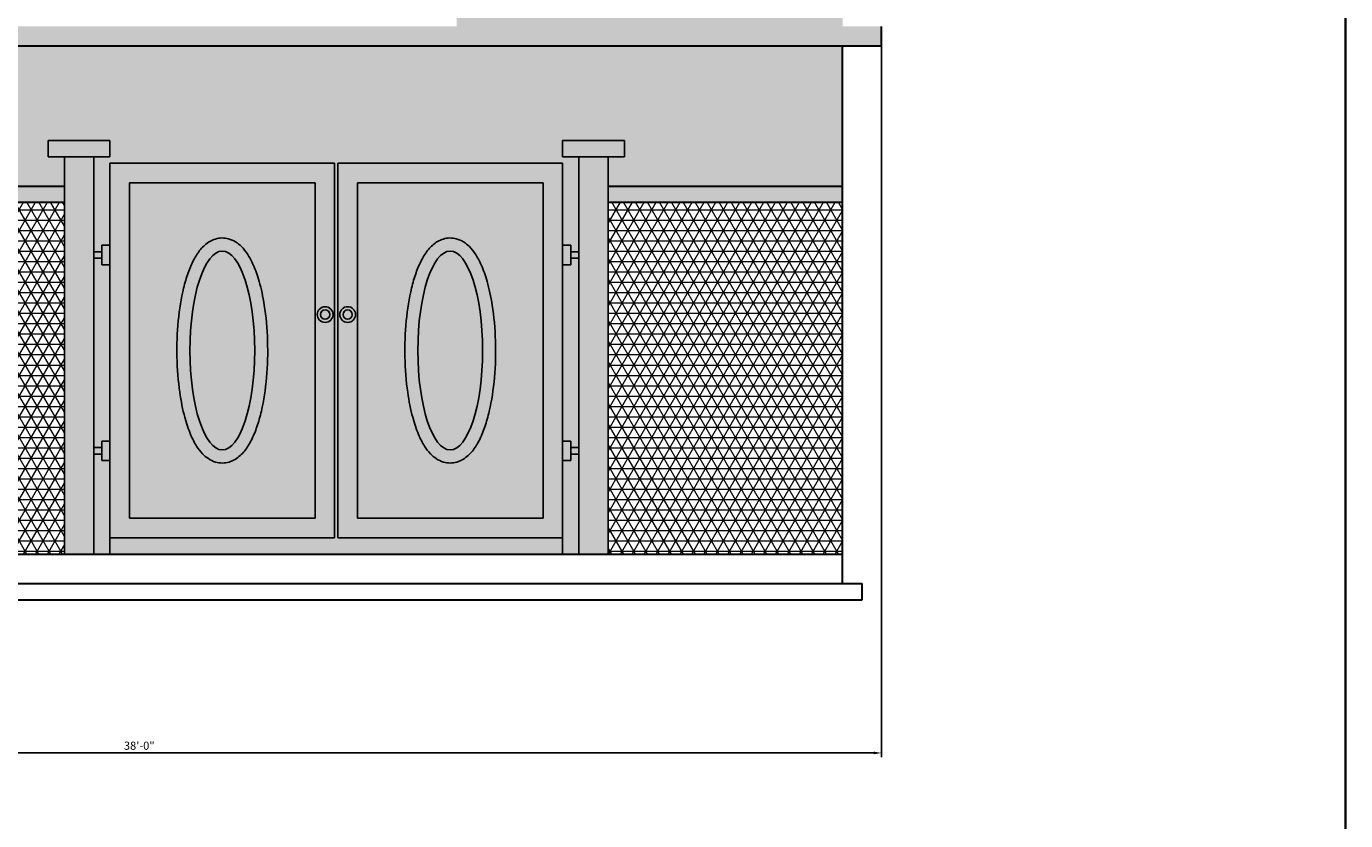
# Model space of a CAD drawing. Units: inches. Extents: x 2391 to 16591, y 7259 to 10239.
# Tile 12 of 27: x 3749 to 4154, y 7502 to 7746. Entities that reach past the tile are written whole.
import ezdxf

# ---------------------------------------------------------------- set-up
doc = ezdxf.new("R2010")
doc.units = ezdxf.units.IN
for name, color, linetype, lineweight in [('A-ANNO-DIMS', 4, 'Continuous', 18), ('A-ANNO-TTLB', 7, 'Continuous', 35), ('A-ELEV', 7, 'Continuous', 30), ('A-ELEV-GATE', 7, 'Continuous', 25), ('A-ELEV-GATE-PATT', 252, 'Continuous', 13), ('A-ELEV-PATT', 8, 'Continuous', 13), ('A-ELEV-SURF-PATT', 253, 'Continuous', 13)]:
    doc.layers.add(name, color=color, linetype=linetype, lineweight=lineweight)
doc.styles.get("Standard").update_dxf_attribs({"font": 'arial.ttf'})
doc.dimstyles.new('ISO-25', dxfattribs={"dimtxt": 2.5, "dimasz": 2.5, "dimexe": 1.25, "dimexo": 0.625, "dimtad": 1, "dimdec": 0, "dimlunit": 3, "dimtxsty": 'Standard', "dimcen": 2.5, "dimadec": 0, "dimazin": 0, "dimtfac": 1, "dimtdec": 0, "dimtmove": 0, "dimatfit": 3, "dimfxl": 1, "dimarcsym": 0})

# ---------------------------------------------------------------- blocks, each defined once
blk = doc.blocks.new('*D91')
at = {"layer": 'A-ANNO-DIMS', "color": 0, "lineweight": -2, "transparency": 16777216}
for p, q in [((3555.71, 7745.56), (3555.71, 7521.88)), ((4011.71, 7745.56), (4011.71, 7521.88)), ((3558.21, 7523.13), (4009.21, 7523.13))]:
    blk.add_line(p, q, dxfattribs=at)
at = {"layer": 'A-ANNO-DIMS', "color": 0, "transparency": 16777216}
for points in [[(3558.21, 7523.55), (3558.21, 7522.71), (3555.71, 7523.13)], [(4009.21, 7523.55), (4009.21, 7522.71), (4011.71, 7523.13)]]:
    blk.add_solid(points, dxfattribs=at)
at = {"layer": 'Defpoints', "color": 0, "transparency": 16777216}
for p in [(3555.71, 7746.18), (4011.71, 7746.18), (4011.71, 7523.13)]:
    blk.add_point(p, dxfattribs=at)
at = {"layer": 'A-ANNO-DIMS', "color": 0, "transparency": 16777216, "insert": (3783.71, 7525.03), "char_height": 2.5, "attachment_point": 5}
blk.add_mtext('38\'-0"', dxfattribs=at)
blk = doc.blocks.new('*D92')
at = {"layer": 'A-ANNO-DIMS', "color": 0, "lineweight": -2, "transparency": 16777216}
for p, q in [((3777.58, 8333.18), (3507.41, 8333.18)), ((3508.66, 7572.68), (3508.66, 8330.68)), ((3561.08, 7570.18), (3507.41, 7570.18))]:
    blk.add_line(p, q, dxfattribs=at)
at = {"layer": 'A-ANNO-DIMS', "color": 0, "transparency": 16777216}
for points in [[(3508.24, 8330.68), (3509.08, 8330.68), (3508.66, 8333.18)], [(3508.24, 7572.68), (3509.08, 7572.68), (3508.66, 7570.18)]]:
    blk.add_solid(points, dxfattribs=at)
at = {"layer": 'Defpoints', "color": 0, "transparency": 16777216}
for p in [(3508.66, 8333.18), (3778.21, 8333.18), (3561.71, 7570.18)]:
    blk.add_point(p, dxfattribs=at)
at = {"layer": 'A-ANNO-DIMS', "color": 0, "transparency": 16777216, "insert": (3506.76, 7951.68), "char_height": 2.5, "attachment_point": 5, "rotation": 90}
blk.add_mtext('63\'-7"', dxfattribs=at)

msp = doc.modelspace()

# ---------------------------------------------------------------- hatches: boundary and pattern name
at = {"layer": 'A-ELEV-GATE-PATT'}
h = msp.add_hatch(color=256, dxfattribs=at)
h.dxf.hatch_style = 1
h.paths.add_polyline_path([(3760.71, 7584.18), (3769.71, 7584.18), (3769.71, 7706.18), (3760.71, 7706.18)])
h.paths.add_polyline_path([(3927.71, 7706.18), (3918.71, 7706.18), (3918.71, 7584.18), (3927.71, 7584.18)])
h = msp.add_hatch(color=256, dxfattribs=at)
h.dxf.hatch_style = 1
h.paths.add_polyline_path([(3774.71, 7589.18), (3843.71, 7589.18), (3843.71, 7704.18), (3774.71, 7704.18)])
h.paths.add_polyline_path([(3780.71, 7698.18), (3837.71, 7698.18), (3837.71, 7595.18), (3780.71, 7595.18)], flags=16)
edge = h.paths.add_edge_path(flags=0)
edge.add_spline(control_points=[(3809.21, 7612.14), (3809.91, 7612.14), (3810.62, 7612.25), (3811.94, 7612.64), (3812.56, 7612.92), (3813.7, 7613.59), (3814.21, 7613.98), (3815.17, 7614.84), (3815.6, 7615.31), (3816.82, 7616.8), (3817.52, 7617.93), (3818.78, 7620.42), (3819.34, 7621.79), (3820.36, 7624.75), (3820.81, 7626.35), (3821.94, 7631.21), (3822.47, 7634.72), (3823.12, 7642.05), (3823.22, 7645.88), (3822.99, 7653.42), (3822.66, 7657.13), (3821.7, 7663.19), (3821.18, 7665.65), (3820.01, 7669.74), (3819.41, 7671.44), (3818.18, 7674.2), (3817.58, 7675.32), (3816.36, 7677.16), (3815.76, 7677.91), (3814.54, 7679.12), (3813.94, 7679.61), (3812.61, 7680.43), (3811.87, 7680.77), (3810.43, 7681.15), (3809.76, 7681.23), (3808.41, 7681.21), (3807.74, 7681.1), (3806.48, 7680.72), (3805.88, 7680.46), (3804.79, 7679.82), (3804.29, 7679.45), (3803.37, 7678.64), (3802.95, 7678.2), (3801.74, 7676.76), (3801.04, 7675.67), (3799.78, 7673.25), (3799.21, 7671.92), (3798.19, 7669.04), (3797.74, 7667.49), (3796.6, 7662.76), (3796.04, 7659.34), (3795.35, 7652.17), (3795.21, 7648.41), (3795.36, 7640.98), (3795.65, 7637.3), (3796.53, 7631.12), (3797.05, 7628.54), (3798.2, 7624.26), (3798.8, 7622.48), (3800.03, 7619.59), (3800.63, 7618.41), (3801.85, 7616.48), (3802.45, 7615.7), (3803.67, 7614.43), (3804.26, 7613.91), (3805.6, 7613.04), (3806.34, 7612.67), (3807.81, 7612.25), (3808.51, 7612.14), (3809.21, 7612.14)], knot_values=[0, 0, 0, 0, 0.095196, 0.095196, 0.190392, 0.190392, 0.285588, 0.285588, 0.380784, 0.380784, 0.570897, 0.570897, 0.76101, 0.76101, 0.951123, 0.951123, 1.307609, 1.307609, 1.664096, 1.664096, 2.020583, 2.020583, 2.290036, 2.290036, 2.5108, 2.5108, 2.687191, 2.687191, 2.829292, 2.829292, 2.942747, 2.942747, 3.056202, 3.056202, 3.147245, 3.147245, 3.238288, 3.238288, 3.329331, 3.329331, 3.420374, 3.420374, 3.511418, 3.511418, 3.698581, 3.698581, 3.885745, 3.885745, 4.072908, 4.072908, 4.42383, 4.42383, 4.774752, 4.774752, 5.125674, 5.125674, 5.403289, 5.403289, 5.629501, 5.629501, 5.810378, 5.810378, 5.956164, 5.956164, 6.072402, 6.072402, 6.18864, 6.18864, 6.283185, 6.283185, 6.283185, 6.283185], degree=3, periodic=0)
edge = h.paths.add_edge_path(flags=0)
edge.add_ellipse((3809.21, 7646.68), major_axis=(0, -30.54), ratio=0.325581, start_angle=0, end_angle=360)
h.paths.add_polyline_path([(3842.21, 7657.71, -1), (3839.37, 7657.71, -1)], flags=16)
h.paths.add_polyline_path([(3844.71, 7589.18), (3913.71, 7589.18), (3913.71, 7704.18), (3844.71, 7704.18)])
h.paths.add_polyline_path([(3850.71, 7698.18), (3907.71, 7698.18), (3907.71, 7595.18), (3850.71, 7595.18)], flags=16)
edge = h.paths.add_edge_path(flags=0)
edge.add_spline(control_points=[(3879.21, 7612.14), (3879.91, 7612.14), (3880.62, 7612.25), (3881.94, 7612.64), (3882.56, 7612.92), (3883.7, 7613.59), (3884.21, 7613.98), (3885.17, 7614.84), (3885.6, 7615.31), (3886.82, 7616.8), (3887.52, 7617.93), (3888.78, 7620.42), (3889.34, 7621.79), (3890.36, 7624.75), (3890.81, 7626.35), (3891.94, 7631.21), (3892.47, 7634.72), (3893.12, 7642.05), (3893.22, 7645.88), (3892.99, 7653.42), (3892.66, 7657.13), (3891.7, 7663.19), (3891.18, 7665.65), (3890.01, 7669.74), (3889.41, 7671.44), (3888.18, 7674.2), (3887.58, 7675.32), (3886.36, 7677.16), (3885.76, 7677.91), (3884.54, 7679.12), (3883.94, 7679.61), (3882.61, 7680.43), (3881.87, 7680.77), (3880.43, 7681.15), (3879.76, 7681.23), (3878.41, 7681.21), (3877.74, 7681.1), (3876.48, 7680.72), (3875.88, 7680.46), (3874.79, 7679.82), (3874.29, 7679.45), (3873.37, 7678.64), (3872.95, 7678.2), (3871.74, 7676.76), (3871.04, 7675.67), (3869.78, 7673.25), (3869.21, 7671.92), (3868.19, 7669.04), (3867.74, 7667.49), (3866.6, 7662.76), (3866.04, 7659.34), (3865.35, 7652.17), (3865.21, 7648.41), (3865.36, 7640.98), (3865.65, 7637.3), (3866.53, 7631.12), (3867.05, 7628.54), (3868.2, 7624.26), (3868.8, 7622.48), (3870.03, 7619.59), (3870.63, 7618.41), (3871.85, 7616.48), (3872.45, 7615.7), (3873.67, 7614.43), (3874.26, 7613.91), (3875.6, 7613.04), (3876.34, 7612.67), (3877.81, 7612.25), (3878.51, 7612.14), (3879.21, 7612.14)], knot_values=[0, 0, 0, 0, 0.095196, 0.095196, 0.190392, 0.190392, 0.285588, 0.285588, 0.380784, 0.380784, 0.570897, 0.570897, 0.76101, 0.76101, 0.951123, 0.951123, 1.307609, 1.307609, 1.664096, 1.664096, 2.020583, 2.020583, 2.290036, 2.290036, 2.5108, 2.5108, 2.687191, 2.687191, 2.829292, 2.829292, 2.942747, 2.942747, 3.056202, 3.056202, 3.147245, 3.147245, 3.238288, 3.238288, 3.329331, 3.329331, 3.420374, 3.420374, 3.511418, 3.511418, 3.698581, 3.698581, 3.885745, 3.885745, 4.072908, 4.072908, 4.42383, 4.42383, 4.774752, 4.774752, 5.125674, 5.125674, 5.403289, 5.403289, 5.629501, 5.629501, 5.810378, 5.810378, 5.956164, 5.956164, 6.072402, 6.072402, 6.18864, 6.18864, 6.283185, 6.283185, 6.283185, 6.283185], degree=3, periodic=0)
edge = h.paths.add_edge_path(flags=0)
edge.add_ellipse((3879.21, 7646.68), major_axis=(0, -30.54), ratio=0.325581, start_angle=0, end_angle=360)
h.paths.add_polyline_path([(3850.12, 7657.71, -1), (3845.29, 7657.71, -1)], flags=16)
h.paths.add_polyline_path([(3849.12, 7657.71, -1), (3846.29, 7657.71, -1)], flags=0)
h = msp.add_hatch(color=256, dxfattribs=at)
h.dxf.hatch_style = 1
h.paths.add_polyline_path([(3780.71, 7698.18), (3780.71, 7595.18), (3837.71, 7595.18), (3837.71, 7698.18)])
edge = h.paths.add_edge_path(flags=16)
edge.add_spline(control_points=[(3809.21, 7612.14), (3809.91, 7612.14), (3810.62, 7612.25), (3811.94, 7612.64), (3812.56, 7612.92), (3813.7, 7613.59), (3814.21, 7613.98), (3815.17, 7614.84), (3815.6, 7615.31), (3816.82, 7616.8), (3817.52, 7617.93), (3818.78, 7620.42), (3819.34, 7621.79), (3820.36, 7624.75), (3820.81, 7626.35), (3821.94, 7631.21), (3822.47, 7634.72), (3823.12, 7642.05), (3823.22, 7645.88), (3822.99, 7653.42), (3822.66, 7657.13), (3821.7, 7663.19), (3821.18, 7665.65), (3820.01, 7669.74), (3819.41, 7671.44), (3818.18, 7674.2), (3817.58, 7675.32), (3816.36, 7677.16), (3815.76, 7677.91), (3814.54, 7679.12), (3813.94, 7679.61), (3812.61, 7680.43), (3811.87, 7680.77), (3810.43, 7681.15), (3809.76, 7681.23), (3808.41, 7681.21), (3807.74, 7681.1), (3806.48, 7680.72), (3805.88, 7680.46), (3804.79, 7679.82), (3804.29, 7679.45), (3803.37, 7678.64), (3802.95, 7678.2), (3801.74, 7676.76), (3801.04, 7675.67), (3799.78, 7673.25), (3799.21, 7671.92), (3798.19, 7669.04), (3797.74, 7667.49), (3796.6, 7662.76), (3796.04, 7659.34), (3795.35, 7652.17), (3795.21, 7648.41), (3795.36, 7640.98), (3795.65, 7637.3), (3796.53, 7631.12), (3797.05, 7628.54), (3798.2, 7624.26), (3798.8, 7622.48), (3800.03, 7619.59), (3800.63, 7618.41), (3801.85, 7616.48), (3802.45, 7615.7), (3803.67, 7614.43), (3804.26, 7613.91), (3805.6, 7613.04), (3806.34, 7612.67), (3807.81, 7612.25), (3808.51, 7612.14), (3809.21, 7612.14)], knot_values=[0, 0, 0, 0, 0.095196, 0.095196, 0.190392, 0.190392, 0.285588, 0.285588, 0.380784, 0.380784, 0.570897, 0.570897, 0.76101, 0.76101, 0.951123, 0.951123, 1.307609, 1.307609, 1.664096, 1.664096, 2.020583, 2.020583, 2.290036, 2.290036, 2.5108, 2.5108, 2.687191, 2.687191, 2.829292, 2.829292, 2.942747, 2.942747, 3.056202, 3.056202, 3.147245, 3.147245, 3.238288, 3.238288, 3.329331, 3.329331, 3.420374, 3.420374, 3.511418, 3.511418, 3.698581, 3.698581, 3.885745, 3.885745, 4.072908, 4.072908, 4.42383, 4.42383, 4.774752, 4.774752, 5.125674, 5.125674, 5.403289, 5.403289, 5.629501, 5.629501, 5.810378, 5.810378, 5.956164, 5.956164, 6.072402, 6.072402, 6.18864, 6.18864, 6.283185, 6.283185, 6.283185, 6.283185], degree=3, periodic=0)
edge = h.paths.add_edge_path(flags=0)
edge.add_ellipse((3809.21, 7646.68), major_axis=(0, -30.54), ratio=0.325581, start_angle=0, end_angle=360)
h.paths.add_polyline_path([(3850.71, 7698.18), (3850.71, 7595.18), (3907.71, 7595.18), (3907.71, 7698.18)])
edge = h.paths.add_edge_path(flags=16)
edge.add_spline(control_points=[(3879.21, 7612.14), (3879.91, 7612.14), (3880.62, 7612.25), (3881.94, 7612.64), (3882.56, 7612.92), (3883.7, 7613.59), (3884.21, 7613.98), (3885.17, 7614.84), (3885.6, 7615.31), (3886.82, 7616.8), (3887.52, 7617.93), (3888.78, 7620.42), (3889.34, 7621.79), (3890.36, 7624.75), (3890.81, 7626.35), (3891.94, 7631.21), (3892.47, 7634.72), (3893.12, 7642.05), (3893.22, 7645.88), (3892.99, 7653.42), (3892.66, 7657.13), (3891.7, 7663.19), (3891.18, 7665.65), (3890.01, 7669.74), (3889.41, 7671.44), (3888.18, 7674.2), (3887.58, 7675.32), (3886.36, 7677.16), (3885.76, 7677.91), (3884.54, 7679.12), (3883.94, 7679.61), (3882.61, 7680.43), (3881.87, 7680.77), (3880.43, 7681.15), (3879.76, 7681.23), (3878.41, 7681.21), (3877.74, 7681.1), (3876.48, 7680.72), (3875.88, 7680.46), (3874.79, 7679.82), (3874.29, 7679.45), (3873.37, 7678.64), (3872.95, 7678.2), (3871.74, 7676.76), (3871.04, 7675.67), (3869.78, 7673.25), (3869.21, 7671.92), (3868.19, 7669.04), (3867.74, 7667.49), (3866.6, 7662.76), (3866.04, 7659.34), (3865.35, 7652.17), (3865.21, 7648.41), (3865.36, 7640.98), (3865.65, 7637.3), (3866.53, 7631.12), (3867.05, 7628.54), (3868.2, 7624.26), (3868.8, 7622.48), (3870.03, 7619.59), (3870.63, 7618.41), (3871.85, 7616.48), (3872.45, 7615.7), (3873.67, 7614.43), (3874.26, 7613.91), (3875.6, 7613.04), (3876.34, 7612.67), (3877.81, 7612.25), (3878.51, 7612.14), (3879.21, 7612.14)], knot_values=[0, 0, 0, 0, 0.095196, 0.095196, 0.190392, 0.190392, 0.285588, 0.285588, 0.380784, 0.380784, 0.570897, 0.570897, 0.76101, 0.76101, 0.951123, 0.951123, 1.307609, 1.307609, 1.664096, 1.664096, 2.020583, 2.020583, 2.290036, 2.290036, 2.5108, 2.5108, 2.687191, 2.687191, 2.829292, 2.829292, 2.942747, 2.942747, 3.056202, 3.056202, 3.147245, 3.147245, 3.238288, 3.238288, 3.329331, 3.329331, 3.420374, 3.420374, 3.511418, 3.511418, 3.698581, 3.698581, 3.885745, 3.885745, 4.072908, 4.072908, 4.42383, 4.42383, 4.774752, 4.774752, 5.125674, 5.125674, 5.403289, 5.403289, 5.629501, 5.629501, 5.810378, 5.810378, 5.956164, 5.956164, 6.072402, 6.072402, 6.18864, 6.18864, 6.283185, 6.283185, 6.283185, 6.283185], degree=3, periodic=0)
edge = h.paths.add_edge_path(flags=0)
edge.add_ellipse((3879.21, 7646.68), major_axis=(0, -30.54), ratio=0.325581, start_angle=0, end_angle=360)
h = msp.add_hatch(color=256, dxfattribs=at)
h.dxf.hatch_style = 1
h.paths.add_polyline_path([(3774.71, 7679.02), (3772.21, 7679.02), (3772.21, 7673.02), (3774.71, 7673.02)])
h.paths.add_polyline_path([(3772.21, 7677.02), (3769.71, 7677.02), (3769.71, 7675.02), (3772.21, 7675.02)])
h.paths.add_polyline_path([(3772.21, 7616.89), (3769.71, 7616.89), (3769.71, 7614.89), (3772.21, 7614.89)])
h.paths.add_polyline_path([(3774.71, 7618.89), (3772.21, 7618.89), (3772.21, 7612.89), (3774.71, 7612.89)])
h.paths.add_polyline_path([(3918.71, 7677.02), (3916.21, 7677.02), (3916.21, 7675.02), (3918.71, 7675.02)])
h.paths.add_polyline_path([(3916.21, 7679.02), (3913.71, 7679.02), (3913.71, 7673.02), (3916.21, 7673.02)])
h.paths.add_polyline_path([(3916.21, 7618.89), (3913.71, 7618.89), (3913.71, 7612.89), (3916.21, 7612.89)])
h.paths.add_polyline_path([(3918.71, 7616.89), (3916.21, 7616.89), (3916.21, 7614.89), (3918.71, 7614.89)])
h = msp.add_hatch(color=256, dxfattribs=at)
h.dxf.hatch_style = 1
edge = h.paths.add_edge_path()
edge.add_spline(control_points=[(3809.21, 7612.14), (3809.91, 7612.14), (3810.62, 7612.25), (3811.94, 7612.64), (3812.56, 7612.92), (3813.7, 7613.59), (3814.21, 7613.98), (3815.17, 7614.84), (3815.6, 7615.31), (3816.82, 7616.8), (3817.52, 7617.93), (3818.78, 7620.42), (3819.34, 7621.79), (3820.36, 7624.75), (3820.81, 7626.35), (3821.94, 7631.21), (3822.47, 7634.72), (3823.12, 7642.05), (3823.22, 7645.88), (3822.99, 7653.42), (3822.66, 7657.13), (3821.7, 7663.19), (3821.18, 7665.65), (3820.01, 7669.74), (3819.41, 7671.44), (3818.18, 7674.2), (3817.58, 7675.32), (3816.36, 7677.16), (3815.76, 7677.91), (3814.54, 7679.12), (3813.94, 7679.61), (3812.61, 7680.43), (3811.87, 7680.77), (3810.43, 7681.15), (3809.76, 7681.23), (3808.41, 7681.21), (3807.74, 7681.1), (3806.48, 7680.72), (3805.88, 7680.46), (3804.79, 7679.82), (3804.29, 7679.45), (3803.37, 7678.64), (3802.95, 7678.2), (3801.74, 7676.76), (3801.04, 7675.67), (3799.78, 7673.25), (3799.21, 7671.92), (3798.19, 7669.04), (3797.74, 7667.49), (3796.6, 7662.76), (3796.04, 7659.34), (3795.35, 7652.17), (3795.21, 7648.41), (3795.36, 7640.98), (3795.65, 7637.3), (3796.53, 7631.12), (3797.05, 7628.54), (3798.2, 7624.26), (3798.8, 7622.48), (3800.03, 7619.59), (3800.63, 7618.41), (3801.85, 7616.48), (3802.45, 7615.7), (3803.67, 7614.43), (3804.26, 7613.91), (3805.6, 7613.04), (3806.34, 7612.67), (3807.81, 7612.25), (3808.51, 7612.14), (3809.21, 7612.14)], knot_values=[0, 0, 0, 0, 0.095196, 0.095196, 0.190392, 0.190392, 0.285588, 0.285588, 0.380784, 0.380784, 0.570897, 0.570897, 0.76101, 0.76101, 0.951123, 0.951123, 1.307609, 1.307609, 1.664096, 1.664096, 2.020583, 2.020583, 2.290036, 2.290036, 2.5108, 2.5108, 2.687191, 2.687191, 2.829292, 2.829292, 2.942747, 2.942747, 3.056202, 3.056202, 3.147245, 3.147245, 3.238288, 3.238288, 3.329331, 3.329331, 3.420374, 3.420374, 3.511418, 3.511418, 3.698581, 3.698581, 3.885745, 3.885745, 4.072908, 4.072908, 4.42383, 4.42383, 4.774752, 4.774752, 5.125674, 5.125674, 5.403289, 5.403289, 5.629501, 5.629501, 5.810378, 5.810378, 5.956164, 5.956164, 6.072402, 6.072402, 6.18864, 6.18864, 6.283185, 6.283185, 6.283185, 6.283185], degree=3, periodic=0)
edge = h.paths.add_edge_path(flags=16)
edge.add_ellipse((3809.21, 7646.68), major_axis=(0, -30.54), ratio=0.325581, start_angle=0, end_angle=360)
edge = h.paths.add_edge_path()
edge.add_spline(control_points=[(3879.21, 7612.14), (3879.91, 7612.14), (3880.62, 7612.25), (3881.94, 7612.64), (3882.56, 7612.92), (3883.7, 7613.59), (3884.21, 7613.98), (3885.17, 7614.84), (3885.6, 7615.31), (3886.82, 7616.8), (3887.52, 7617.93), (3888.78, 7620.42), (3889.34, 7621.79), (3890.36, 7624.75), (3890.81, 7626.35), (3891.94, 7631.21), (3892.47, 7634.72), (3893.12, 7642.05), (3893.22, 7645.88), (3892.99, 7653.42), (3892.66, 7657.13), (3891.7, 7663.19), (3891.18, 7665.65), (3890.01, 7669.74), (3889.41, 7671.44), (3888.18, 7674.2), (3887.58, 7675.32), (3886.36, 7677.16), (3885.76, 7677.91), (3884.54, 7679.12), (3883.94, 7679.61), (3882.61, 7680.43), (3881.87, 7680.77), (3880.43, 7681.15), (3879.76, 7681.23), (3878.41, 7681.21), (3877.74, 7681.1), (3876.48, 7680.72), (3875.88, 7680.46), (3874.79, 7679.82), (3874.29, 7679.45), (3873.37, 7678.64), (3872.95, 7678.2), (3871.74, 7676.76), (3871.04, 7675.67), (3869.78, 7673.25), (3869.21, 7671.92), (3868.19, 7669.04), (3867.74, 7667.49), (3866.6, 7662.76), (3866.04, 7659.34), (3865.35, 7652.17), (3865.21, 7648.41), (3865.36, 7640.98), (3865.65, 7637.3), (3866.53, 7631.12), (3867.05, 7628.54), (3868.2, 7624.26), (3868.8, 7622.48), (3870.03, 7619.59), (3870.63, 7618.41), (3871.85, 7616.48), (3872.45, 7615.7), (3873.67, 7614.43), (3874.26, 7613.91), (3875.6, 7613.04), (3876.34, 7612.67), (3877.81, 7612.25), (3878.51, 7612.14), (3879.21, 7612.14)], knot_values=[0, 0, 0, 0, 0.095196, 0.095196, 0.190392, 0.190392, 0.285588, 0.285588, 0.380784, 0.380784, 0.570897, 0.570897, 0.76101, 0.76101, 0.951123, 0.951123, 1.307609, 1.307609, 1.664096, 1.664096, 2.020583, 2.020583, 2.290036, 2.290036, 2.5108, 2.5108, 2.687191, 2.687191, 2.829292, 2.829292, 2.942747, 2.942747, 3.056202, 3.056202, 3.147245, 3.147245, 3.238288, 3.238288, 3.329331, 3.329331, 3.420374, 3.420374, 3.511418, 3.511418, 3.698581, 3.698581, 3.885745, 3.885745, 4.072908, 4.072908, 4.42383, 4.42383, 4.774752, 4.774752, 5.125674, 5.125674, 5.403289, 5.403289, 5.629501, 5.629501, 5.810378, 5.810378, 5.956164, 5.956164, 6.072402, 6.072402, 6.18864, 6.18864, 6.283185, 6.283185, 6.283185, 6.283185], degree=3, periodic=0)
edge = h.paths.add_edge_path(flags=16)
edge.add_ellipse((3879.21, 7646.68), major_axis=(0, -30.54), ratio=0.325581, start_angle=0, end_angle=360)
h = msp.add_hatch(color=256, dxfattribs=at)
h.dxf.hatch_style = 1
edge = h.paths.add_edge_path()
edge.add_ellipse((3809.21, 7646.68), major_axis=(0, -30.54), ratio=0.325581, start_angle=0, end_angle=360)
edge = h.paths.add_edge_path()
edge.add_ellipse((3879.21, 7646.68), major_axis=(0, -30.54), ratio=0.325581, start_angle=0, end_angle=360)
h = msp.add_hatch(color=256, dxfattribs=at)
h.dxf.hatch_style = 1
h.paths.add_polyline_path([(3843.21, 7657.71, 1), (3838.37, 7657.71, 1)])
h.paths.add_polyline_path([(3842.21, 7657.71, 1), (3839.37, 7657.71, 1)], flags=16)
h.paths.add_polyline_path([(3850.12, 7657.71, 1), (3845.29, 7657.71, 1)])
h.paths.add_polyline_path([(3849.12, 7657.71, 1), (3846.29, 7657.71, 1)], flags=16)
h = msp.add_hatch(color=256, dxfattribs=at)
h.dxf.hatch_style = 1
h.paths.add_polyline_path([(3842.21, 7657.71, 1), (3839.37, 7657.71, 1)])
h.paths.add_polyline_path([(3849.12, 7657.71, 1), (3846.29, 7657.71, 1)])
at = {"layer": 'A-ELEV-PATT'}
h = msp.add_hatch(dxfattribs=at)
h.set_pattern_fill('BRSTONE', color=256)
h.paths.add_polyline_path([(3999.71, 8226.18), (3881.21, 8226.18), (3881.21, 8070.18), (3999.71, 8070.18)])
h.paths.add_polyline_path([(3956.96, 8118.18), (3914.96, 8118.18), (3914.96, 8172.18), (3956.96, 8172.18)], flags=16)
h.paths.add_polyline_path([(3953.96, 8121.18), (3917.96, 8121.18), (3917.96, 8169.18), (3953.96, 8169.18)], flags=0)
h.paths.add_polyline_path([(3999.71, 8064.18), (3881.21, 8064.18), (3881.21, 7908.18), (3999.71, 7908.18)])
h.paths.add_polyline_path([(3956.96, 7956.18), (3914.96, 7956.18), (3914.96, 8010.18), (3956.96, 8010.18)], flags=16)
h.paths.add_polyline_path([(3953.96, 7959.18), (3917.96, 7959.18), (3917.96, 8007.18), (3953.96, 8007.18)], flags=0)
h.paths.add_polyline_path([(3999.71, 7902.18), (3881.21, 7902.18), (3881.21, 7746.18), (3999.71, 7746.18)])
h.paths.add_polyline_path([(3956.96, 7794.18), (3914.96, 7794.18), (3914.96, 7848.18), (3956.96, 7848.18)], flags=16)
h.paths.add_polyline_path([(3953.96, 7797.18), (3917.96, 7797.18), (3917.96, 7845.18), (3953.96, 7845.18)], flags=0)
h.paths.add_polyline_path([(3999.71, 7740.18), (3567.71, 7740.18), (3567.71, 7697.18), (3760.71, 7697.18), (3760.71, 7706.18), (3755.71, 7706.18), (3755.71, 7711.18), (3774.71, 7711.18), (3774.71, 7706.18), (3769.71, 7706.18), (3769.71, 7677.02), (3772.21, 7677.02), (3772.21, 7679.02), (3774.71, 7679.02), (3774.71, 7704.18), (3843.71, 7704.18), (3843.71, 7589.18), (3774.71, 7589.18), (3774.71, 7584.18), (3913.71, 7584.18), (3913.71, 7589.18), (3844.71, 7589.18), (3844.71, 7704.18), (3913.71, 7704.18), (3913.71, 7679.02), (3916.21, 7679.02), (3916.21, 7677.02), (3918.71, 7677.02), (3918.71, 7706.18), (3913.71, 7706.18), (3913.71, 7711.18), (3932.71, 7711.18), (3932.71, 7706.18), (3927.71, 7706.18), (3927.71, 7697.18), (3999.71, 7697.18)])
h.paths.add_polyline_path([(3918.71, 7675.02), (3916.21, 7675.02), (3916.21, 7673.02), (3913.71, 7673.02), (3913.71, 7618.89), (3916.21, 7618.89), (3916.21, 7616.89), (3918.71, 7616.89)], flags=17)
h.paths.add_polyline_path([(3918.71, 7614.89), (3916.21, 7614.89), (3916.21, 7612.89), (3913.71, 7612.89), (3913.71, 7584.18), (3918.71, 7584.18)], flags=17)
h.paths.add_polyline_path([(3774.71, 7673.02), (3772.21, 7673.02), (3772.21, 7675.02), (3769.71, 7675.02), (3769.71, 7616.89), (3772.21, 7616.89), (3772.21, 7618.89), (3774.71, 7618.89)], flags=17)
h.paths.add_polyline_path([(3774.71, 7612.89), (3772.21, 7612.89), (3772.21, 7614.89), (3769.71, 7614.89), (3769.71, 7584.18), (3774.71, 7584.18), (3774.71, 7589.18)], flags=17)
h = msp.add_hatch(dxfattribs=at)
h.set_pattern_fill('NET3', color=256)
h.paths.add_polyline_path([(3760.71, 7692.18), (3567.71, 7692.18), (3567.71, 7584.18), (3760.71, 7584.18)])
h.paths.add_polyline_path([(3999.71, 7692.18), (3927.71, 7692.18), (3927.71, 7584.18), (3999.71, 7584.18)])
at = {"layer": 'A-ELEV-SURF-PATT'}
h = msp.add_hatch(color=256, dxfattribs=at)
h.dxf.hatch_style = 1
h.paths.add_polyline_path([(4011.71, 7740.18), (4011.71, 7746.18), (3555.71, 7746.18), (3555.71, 7740.18)])
h.paths.add_polyline_path([(4011.71, 7902.18), (4011.71, 7908.18), (3555.71, 7908.18), (3555.71, 7902.18)])
h.paths.add_polyline_path([(4011.71, 8064.18), (4011.71, 8070.18), (3555.71, 8070.18), (3555.71, 8064.18)])
h.paths.add_polyline_path([(3555.71, 8232.18), (3555.71, 8226.18), (4011.71, 8226.18), (4011.71, 8232.18)])
h.paths.add_polyline_path([(3778.21, 8333.18), (3778.21, 8328.18), (3978.71, 8328.18), (3978.71, 8333.18)])
h = msp.add_hatch(color=256, dxfattribs=at)
h.dxf.hatch_style = 1
h.paths.add_polyline_path([(3760.71, 7692.18), (3760.71, 7697.18), (3567.71, 7697.18), (3567.71, 7692.18)])
h.paths.add_polyline_path([(3755.71, 7711.18), (3755.71, 7706.18), (3774.71, 7706.18), (3774.71, 7711.18)])
h.paths.add_polyline_path([(3913.71, 7711.18), (3913.71, 7706.18), (3932.71, 7706.18), (3932.71, 7711.18)])
h.paths.add_polyline_path([(3927.71, 7697.18), (3927.71, 7692.18), (3999.71, 7692.18), (3999.71, 7697.18)])

# ---------------------------------------------------------------- linework, layer by layer
at = {"layer": 'A-ANNO-TTLB'}
msp.add_lwpolyline([(2391.28, 10239.38), (4154.2, 10239.38), (4154.2, 7258.54), (2391.28, 7258.54)], close=True, dxfattribs=at)
at = {"layer": 'A-ELEV'}
for p, q in [((4011.71, 7740.18), (4011.71, 7746.18)), ((3555.71, 7740.18), (4011.71, 7740.18)), ((3999.71, 7575.18), (3999.71, 7740.18)), ((3567.71, 7697.18), (3760.71, 7697.18)), ((3927.71, 7697.18), (3999.71, 7697.18)), ((3567.71, 7692.18), (3760.71, 7692.18)), ((3927.71, 7692.18), (3999.71, 7692.18)), ((3567.71, 7584.18), (3999.71, 7584.18)), ((3561.71, 7575.18), (4005.71, 7575.18)), ((4005.71, 7570.18), (4005.71, 7575.18)), ((3561.71, 7570.18), (4005.71, 7570.18))]:
    msp.add_line(p, q, dxfattribs=at)
at = {"layer": 'A-ELEV-GATE'}
for p, q in [((3755.71, 7706.18), (3755.71, 7711.18)), ((3774.71, 7711.18), (3755.71, 7711.18)), ((3774.71, 7706.18), (3774.71, 7711.18)), ((3913.71, 7706.18), (3913.71, 7711.18)), ((3913.71, 7711.18), (3932.71, 7711.18)), ((3932.71, 7706.18), (3932.71, 7711.18)), ((3774.71, 7706.18), (3755.71, 7706.18)), ((3760.71, 7584.18), (3760.71, 7706.18)), ((3769.71, 7584.18), (3769.71, 7706.18)), ((3913.71, 7706.18), (3932.71, 7706.18)), ((3918.71, 7584.18), (3918.71, 7706.18)), ((3927.71, 7584.18), (3927.71, 7706.18)), ((3774.71, 7584.18), (3774.71, 7704.18)), ((3774.71, 7704.18), (3843.71, 7704.18)), ((3843.71, 7704.18), (3843.71, 7589.18)), ((3844.71, 7704.18), (3913.71, 7704.18)), ((3844.71, 7704.18), (3844.71, 7589.18)), ((3913.71, 7584.18), (3913.71, 7704.18)), ((3780.71, 7595.18), (3780.71, 7698.18)), ((3780.71, 7698.18), (3837.71, 7698.18)), ((3837.71, 7698.18), (3837.71, 7595.18)), ((3850.71, 7698.18), (3907.71, 7698.18)), ((3850.71, 7698.18), (3850.71, 7595.18)), ((3907.71, 7595.18), (3907.71, 7698.18)), ((3774.71, 7679.02), (3772.21, 7679.02)), ((3772.21, 7679.02), (3772.21, 7673.02)), ((3913.71, 7679.02), (3916.21, 7679.02)), ((3916.21, 7679.02), (3916.21, 7673.02)), ((3772.21, 7677.02), (3769.71, 7677.02)), ((3772.21, 7675.02), (3769.71, 7675.02)), ((3916.21, 7677.02), (3918.71, 7677.02)), ((3916.21, 7675.02), (3918.71, 7675.02)), ((3774.71, 7673.02), (3772.21, 7673.02)), ((3913.71, 7673.02), (3916.21, 7673.02)), ((3774.71, 7618.89), (3772.21, 7618.89)), ((3772.21, 7618.89), (3772.21, 7612.89)), ((3913.71, 7618.89), (3916.21, 7618.89)), ((3916.21, 7618.89), (3916.21, 7612.89)), ((3772.21, 7616.89), (3769.71, 7616.89)), ((3772.21, 7614.89), (3769.71, 7614.89)), ((3916.21, 7616.89), (3918.71, 7616.89)), ((3916.21, 7614.89), (3918.71, 7614.89)), ((3774.71, 7612.89), (3772.21, 7612.89)), ((3913.71, 7612.89), (3916.21, 7612.89)), ((3780.71, 7595.18), (3837.71, 7595.18)), ((3850.71, 7595.18), (3907.71, 7595.18)), ((3774.71, 7589.18), (3843.71, 7589.18)), ((3844.71, 7589.18), (3913.71, 7589.18))]:
    msp.add_line(p, q, dxfattribs=at)
for centre, radius in [((3840.79, 7657.71), 2.42), ((3840.79, 7657.71), 1.42), ((3847.71, 7657.71), 2.42), ((3847.71, 7657.71), 1.42)]:
    msp.add_circle(centre, radius, dxfattribs=at)
for centre in [(3809.21, 7646.68), (3879.21, 7646.68)]:
    msp.add_ellipse(centre, major_axis=(0, -30.54), ratio=0.325581, dxfattribs=at)
for points in [[(3809.21, 7612.14), (3809.91, 7612.14), (3810.62, 7612.25), (3811.94, 7612.64), (3812.56, 7612.92), (3813.7, 7613.59), (3814.21, 7613.98), (3815.17, 7614.84), (3815.6, 7615.31), (3816.82, 7616.8), (3817.52, 7617.93), (3818.78, 7620.42), (3819.34, 7621.79), (3820.36, 7624.75), (3820.81, 7626.35), (3821.94, 7631.21), (3822.47, 7634.72), (3823.12, 7642.05), (3823.22, 7645.88), (3822.99, 7653.42), (3822.66, 7657.13), (3821.7, 7663.19), (3821.18, 7665.65), (3820.01, 7669.74), (3819.41, 7671.44), (3818.18, 7674.2), (3817.58, 7675.32), (3816.36, 7677.16), (3815.76, 7677.91), (3814.54, 7679.12), (3813.94, 7679.61), (3812.61, 7680.43), (3811.87, 7680.77), (3810.43, 7681.15), (3809.76, 7681.23), (3808.41, 7681.21), (3807.74, 7681.1), (3806.48, 7680.72), (3805.88, 7680.46), (3804.79, 7679.82), (3804.29, 7679.45), (3803.37, 7678.64), (3802.95, 7678.2), (3801.74, 7676.76), (3801.04, 7675.67), (3799.78, 7673.25), (3799.21, 7671.92), (3798.19, 7669.04), (3797.74, 7667.49), (3796.6, 7662.76), (3796.04, 7659.34), (3795.35, 7652.17), (3795.21, 7648.41), (3795.36, 7640.98), (3795.65, 7637.3), (3796.53, 7631.12), (3797.05, 7628.54), (3798.2, 7624.26), (3798.8, 7622.48), (3800.03, 7619.59), (3800.63, 7618.41), (3801.85, 7616.48), (3802.45, 7615.7), (3803.67, 7614.43), (3804.26, 7613.91), (3805.6, 7613.04), (3806.34, 7612.67), (3807.81, 7612.25), (3808.51, 7612.14), (3809.21, 7612.14)], [(3879.21, 7612.14), (3879.91, 7612.14), (3880.62, 7612.25), (3881.94, 7612.64), (3882.56, 7612.92), (3883.7, 7613.59), (3884.21, 7613.98), (3885.17, 7614.84), (3885.6, 7615.31), (3886.82, 7616.8), (3887.52, 7617.93), (3888.78, 7620.42), (3889.34, 7621.79), (3890.36, 7624.75), (3890.81, 7626.35), (3891.94, 7631.21), (3892.47, 7634.72), (3893.12, 7642.05), (3893.22, 7645.88), (3892.99, 7653.42), (3892.66, 7657.13), (3891.7, 7663.19), (3891.18, 7665.65), (3890.01, 7669.74), (3889.41, 7671.44), (3888.18, 7674.2), (3887.58, 7675.32), (3886.36, 7677.16), (3885.76, 7677.91), (3884.54, 7679.12), (3883.94, 7679.61), (3882.61, 7680.43), (3881.87, 7680.77), (3880.43, 7681.15), (3879.76, 7681.23), (3878.41, 7681.21), (3877.74, 7681.1), (3876.48, 7680.72), (3875.88, 7680.46), (3874.79, 7679.82), (3874.29, 7679.45), (3873.37, 7678.64), (3872.95, 7678.2), (3871.74, 7676.76), (3871.04, 7675.67), (3869.78, 7673.25), (3869.21, 7671.92), (3868.19, 7669.04), (3867.74, 7667.49), (3866.6, 7662.76), (3866.04, 7659.34), (3865.35, 7652.17), (3865.21, 7648.41), (3865.36, 7640.98), (3865.65, 7637.3), (3866.53, 7631.12), (3867.05, 7628.54), (3868.2, 7624.26), (3868.8, 7622.48), (3870.03, 7619.59), (3870.63, 7618.41), (3871.85, 7616.48), (3872.45, 7615.7), (3873.67, 7614.43), (3874.26, 7613.91), (3875.6, 7613.04), (3876.34, 7612.67), (3877.81, 7612.25), (3878.51, 7612.14), (3879.21, 7612.14)]]:
    msp.add_open_spline(points, degree=3, knots=[0, 0, 0, 0, 0.095196, 0.095196, 0.190392, 0.190392, 0.285588, 0.285588, 0.380784, 0.380784, 0.570897, 0.570897, 0.76101, 0.76101, 0.951123, 0.951123, 1.307609, 1.307609, 1.664096, 1.664096, 2.020583, 2.020583, 2.290036, 2.290036, 2.5108, 2.5108, 2.687191, 2.687191, 2.829292, 2.829292, 2.942747, 2.942747, 3.056202, 3.056202, 3.147245, 3.147245, 3.238288, 3.238288, 3.329331, 3.329331, 3.420374, 3.420374, 3.511418, 3.511418, 3.698581, 3.698581, 3.885745, 3.885745, 4.072908, 4.072908, 4.42383, 4.42383, 4.774752, 4.774752, 5.125674, 5.125674, 5.403289, 5.403289, 5.629501, 5.629501, 5.810378, 5.810378, 5.956164, 5.956164, 6.072402, 6.072402, 6.18864, 6.18864, 6.283185, 6.283185, 6.283185, 6.283185], dxfattribs=at)

# ---------------------------------------------------------------- dimensions: what is measured, and where the dimension line sits
at = {"layer": 'A-ANNO-DIMS'}
dim = msp.add_linear_dim(base=(3508.66, 8333.18), p1=(3561.71, 7570.18), p2=(3778.21, 8333.18), angle=90, dimstyle='ISO-25', override={"dimdec": 1, "dimlfac": 1, "dimrnd": 0, "dimzin": 1, "dimdsep": 46, "dimlunit": 4, "dimfrac": 2}, dxfattribs=at)
dim.commit()
dim.dimension.update_dxf_attribs({"geometry": '*D92', "text_midpoint": (3506.76, 7951.68)})
dim = msp.add_linear_dim(base=(4011.71, 7523.13), p1=(3555.71, 7746.18), p2=(4011.71, 7746.18), dimstyle='ISO-25', override={"dimdec": 1, "dimlfac": 1, "dimrnd": 0, "dimzin": 1, "dimdsep": 46, "dimlunit": 4, "dimfrac": 2}, dxfattribs=at)
dim.commit()
dim.dimension.update_dxf_attribs({"geometry": '*D91', "text_midpoint": (3783.71, 7525.03)})

doc.saveas('drawing.dxf')
